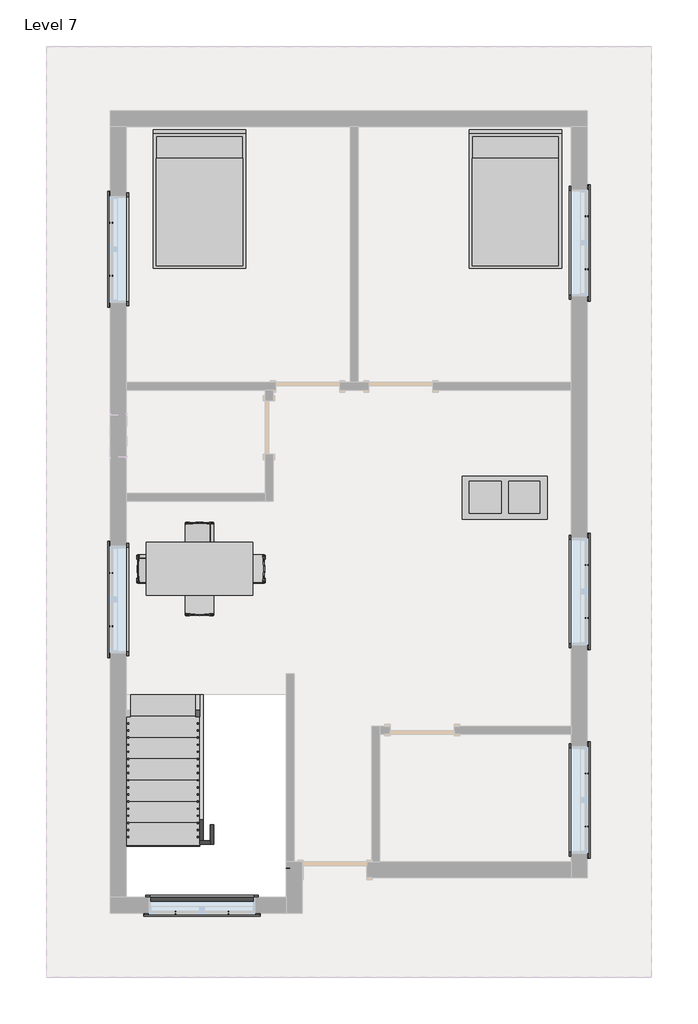
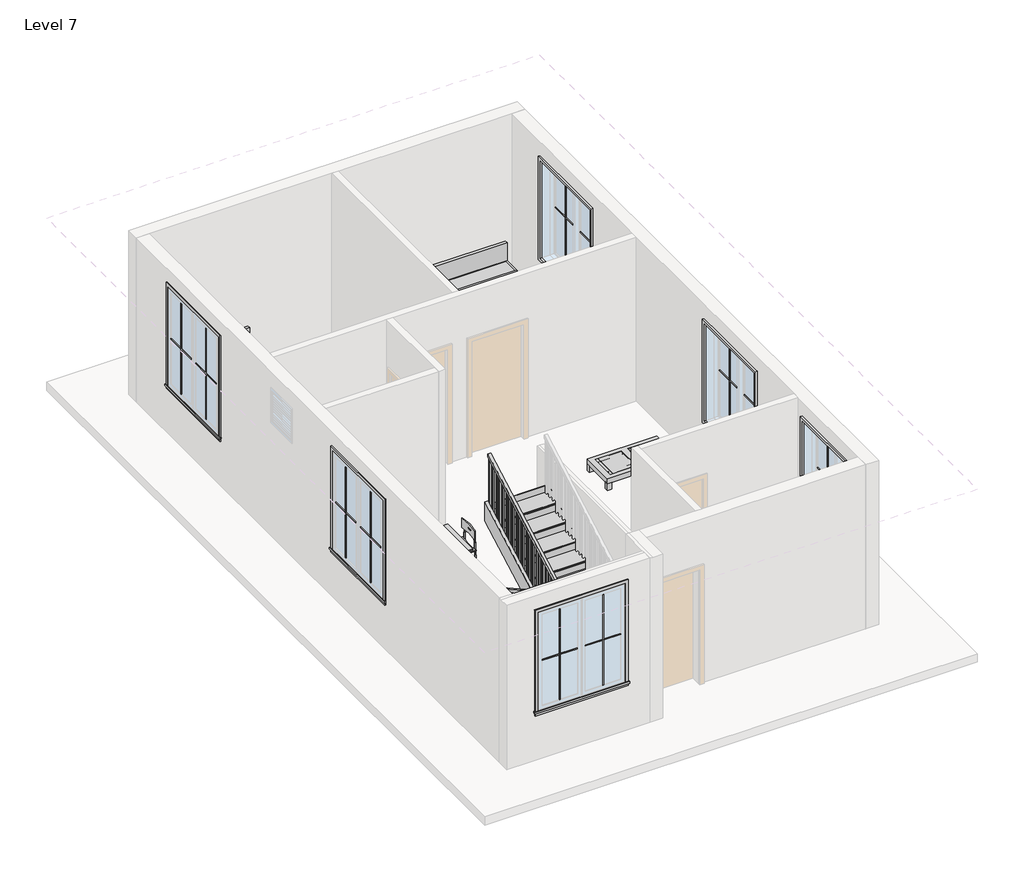
# One storey, part 3 of 3: 25 proxies, 6 members, 3 furniture elements, 1 railing, 1 stair flight.
"""IFC4 building model written with IfcOpenShell, lengths in millimetres."""

from ifc_helpers import new_model, si_unit, frame, origin, place, context, project, spatial, polyline, outline, extrude, faceted_brep, transform, mapped, element, save
from components import muntin_pattern_2x2_muntin_pattern_2x2_f6a80940, muntin_pattern_2x2_muntin_pattern_2x2_09b00a1c, trim_window_exterior_flat_with_sill_698ed857, trim_window_interior_flat_picture_frame_92551a5e, coffee_table_with_brass_mullions_11320_coffee_table_with_5962bef7, bed_17739_bed_17739_15c61121, dining_table_w_chairs_11374_0cdfc61b, stair_flight_c5737279

model = new_model("IFC4")

# Units and contexts
model_context = context("Model", 3, world=origin())
ifc_project = project(units=[si_unit("LENGTHUNIT", "METRE", prefix="MILLI")], contexts=[model_context])

# Site, building, storey
site = spatial("IfcSite", under=ifc_project)
building = spatial("IfcBuilding", under=site)
storey = spatial("IfcBuildingStorey", under=building, Name="Level 7", Elevation=19050.0)

# Proxies
placement = place(None, origin())
muntin_pattern_2x2_muntin_pattern_2x2_shape = muntin_pattern_2x2_muntin_pattern_2x2_f6a80940(model_context)
element("IfcBuildingElementProxy", 1, Name="Muntin Pattern_2x2 : Muntin Pattern_2x2", ObjectType="Muntin Pattern_2x2 : Muntin Pattern_2x2", at=placement, inside=storey, context=model_context, shape_type="MappedRepresentation", body=[
    mapped(muntin_pattern_2x2_muntin_pattern_2x2_shape, transform((-2773.368364, -6686.2830018, 20034.25), x_axis=(-1.0, 0.0, 0.0), y_axis=(0.0, -1.0, 0.0), z_axis=(0.0, 0.0, 1.0))),
])
element("IfcBuildingElementProxy", 2, Name="Muntin Pattern_2x2 : Muntin Pattern_2x2", ObjectType="Muntin Pattern_2x2 : Muntin Pattern_2x2", at=placement, inside=storey, context=model_context, shape_type="MappedRepresentation", body=[
    mapped(muntin_pattern_2x2_muntin_pattern_2x2_shape, transform((2349.494136, -4693.9705018, 20034.25), x_axis=(0.0, -1.0, 0.0), y_axis=(1.0, 0.0, 0.0), z_axis=(0.0, 0.0, 1.0))),
])
element("IfcBuildingElementProxy", 3, Name="Muntin Pattern_2x2 : Muntin Pattern_2x2", ObjectType="Muntin Pattern_2x2 : Muntin Pattern_2x2", at=placement, inside=storey, context=model_context, shape_type="MappedRepresentation", body=[
    mapped(muntin_pattern_2x2_muntin_pattern_2x2_shape, transform((2349.494136, -1712.6455018, 20034.25), x_axis=(0.0, -1.0, 0.0), y_axis=(1.0, 0.0, 0.0), z_axis=(0.0, 0.0, 1.0))),
])
element("IfcBuildingElementProxy", 4, Name="Muntin Pattern_2x2 : Muntin Pattern_2x2", ObjectType="Muntin Pattern_2x2 : Muntin Pattern_2x2", at=placement, inside=storey, context=model_context, shape_type="MappedRepresentation", body=[
    mapped(muntin_pattern_2x2_muntin_pattern_2x2_shape, transform((-4451.355864, -2586.5525081, 20034.25), x_axis=(0.0, 1.0, 0.0), y_axis=(-1.0, 0.0, 0.0), z_axis=(0.0, 0.0, 1.0))),
])
element("IfcBuildingElementProxy", 5, Name="Muntin Pattern_2x2 : Muntin Pattern_2x2", ObjectType="Muntin Pattern_2x2 : Muntin Pattern_2x2", at=placement, inside=storey, context=model_context, shape_type="MappedRepresentation", body=[
    mapped(muntin_pattern_2x2_muntin_pattern_2x2_shape, transform((2349.494136, 3272.1044982, 20034.25), x_axis=(0.0, -1.0, 0.0), y_axis=(1.0, 0.0, 0.0), z_axis=(0.0, 0.0, 1.0))),
])
element("IfcBuildingElementProxy", 6, Name="Muntin Pattern_2x2 : Muntin Pattern_2x2", ObjectType="Muntin Pattern_2x2 : Muntin Pattern_2x2", at=placement, inside=storey, context=model_context, shape_type="MappedRepresentation", body=[
    mapped(muntin_pattern_2x2_muntin_pattern_2x2_shape, transform((-4451.355864, 2421.2162133, 20034.25), x_axis=(0.0, 1.0, 0.0), y_axis=(-1.0, 0.0, 0.0), z_axis=(0.0, 0.0, 1.0))),
])
muntin_pattern_2x2_muntin_pattern_2x2_2_shape = muntin_pattern_2x2_muntin_pattern_2x2_09b00a1c(model_context)
element("IfcBuildingElementProxy", 7, Name="Muntin Pattern_2x2 : Muntin Pattern_2x2", ObjectType="Muntin Pattern_2x2 : Muntin Pattern_2x2", at=placement, inside=storey, context=model_context, shape_type="MappedRepresentation", body=[
    mapped(muntin_pattern_2x2_muntin_pattern_2x2_2_shape, transform((-3532.193364, -6686.2830018, 20034.25), x_axis=(1.0, 0.0, 0.0), y_axis=(0.0, 1.0, 0.0), z_axis=(0.0, 0.0, 1.0))),
])
element("IfcBuildingElementProxy", 8, Name="Muntin Pattern_2x2 : Muntin Pattern_2x2", ObjectType="Muntin Pattern_2x2 : Muntin Pattern_2x2", at=placement, inside=storey, context=model_context, shape_type="MappedRepresentation", body=[
    mapped(muntin_pattern_2x2_muntin_pattern_2x2_2_shape, transform((2349.494136, -5452.7955018, 20034.25), x_axis=(0.0, 1.0, 0.0), y_axis=(-1.0, 0.0, 0.0), z_axis=(0.0, 0.0, 1.0))),
])
element("IfcBuildingElementProxy", 9, Name="Muntin Pattern_2x2 : Muntin Pattern_2x2", ObjectType="Muntin Pattern_2x2 : Muntin Pattern_2x2", at=placement, inside=storey, context=model_context, shape_type="MappedRepresentation", body=[
    mapped(muntin_pattern_2x2_muntin_pattern_2x2_2_shape, transform((2349.494136, -2471.4705018, 20034.25), x_axis=(0.0, 1.0, 0.0), y_axis=(-1.0, 0.0, 0.0), z_axis=(0.0, 0.0, 1.0))),
])
element("IfcBuildingElementProxy", 10, Name="Muntin Pattern_2x2 : Muntin Pattern_2x2", ObjectType="Muntin Pattern_2x2 : Muntin Pattern_2x2", at=placement, inside=storey, context=model_context, shape_type="MappedRepresentation", body=[
    mapped(muntin_pattern_2x2_muntin_pattern_2x2_2_shape, transform((-4451.355864, -1827.7275081, 20034.25), x_axis=(0.0, -1.0, 0.0), y_axis=(1.0, 0.0, 0.0), z_axis=(0.0, 0.0, 1.0))),
])
element("IfcBuildingElementProxy", 11, Name="Muntin Pattern_2x2 : Muntin Pattern_2x2", ObjectType="Muntin Pattern_2x2 : Muntin Pattern_2x2", at=placement, inside=storey, context=model_context, shape_type="MappedRepresentation", body=[
    mapped(muntin_pattern_2x2_muntin_pattern_2x2_2_shape, transform((2349.494136, 2513.2794982, 20034.25), x_axis=(0.0, 1.0, 0.0), y_axis=(-1.0, 0.0, 0.0), z_axis=(0.0, 0.0, 1.0))),
])
element("IfcBuildingElementProxy", 12, Name="Muntin Pattern_2x2 : Muntin Pattern_2x2", ObjectType="Muntin Pattern_2x2 : Muntin Pattern_2x2", at=placement, inside=storey, context=model_context, shape_type="MappedRepresentation", body=[
    mapped(muntin_pattern_2x2_muntin_pattern_2x2_2_shape, transform((-4451.355864, 3180.0412133, 20034.25), x_axis=(0.0, -1.0, 0.0), y_axis=(1.0, 0.0, 0.0), z_axis=(0.0, 0.0, 1.0))),
])
trim_window_exterior_flat_with_sill_shape = trim_window_exterior_flat_with_sill_698ed857(model_context)
element("IfcBuildingElementProxy", 13, Name="Trim-Window-Exterior-Flat : with Sill", ObjectType="Trim-Window-Exterior-Flat : with Sill", at=placement, inside=storey, context=model_context, shape_type="MappedRepresentation", body=[
    mapped(trim_window_exterior_flat_with_sill_shape, transform((-3152.780864, -6695.8080018, 21793.2), x_axis=(1.0, 0.0, 0.0), y_axis=(0.0, 0.0, 1.0), z_axis=(0.0, -1.0, 0.0))),
])
element("IfcBuildingElementProxy", 14, Name="Trim-Window-Exterior-Flat : with Sill", ObjectType="Trim-Window-Exterior-Flat : with Sill", at=placement, inside=storey, context=model_context, shape_type="MappedRepresentation", body=[
    mapped(trim_window_exterior_flat_with_sill_shape, transform((2359.019136, -5073.3830018, 21793.2), x_axis=(0.0, 1.0, 0.0), y_axis=(0.0, 0.0, 1.0), z_axis=(1.0, 0.0, 0.0))),
])
element("IfcBuildingElementProxy", 15, Name="Trim-Window-Exterior-Flat : with Sill", ObjectType="Trim-Window-Exterior-Flat : with Sill", at=placement, inside=storey, context=model_context, shape_type="MappedRepresentation", body=[
    mapped(trim_window_exterior_flat_with_sill_shape, transform((2359.019136, -2092.0580018, 21793.2), x_axis=(0.0, 1.0, 0.0), y_axis=(0.0, 0.0, 1.0), z_axis=(1.0, 0.0, 0.0))),
])
element("IfcBuildingElementProxy", 16, Name="Trim-Window-Exterior-Flat : with Sill", ObjectType="Trim-Window-Exterior-Flat : with Sill", at=placement, inside=storey, context=model_context, shape_type="MappedRepresentation", body=[
    mapped(trim_window_exterior_flat_with_sill_shape, transform((-4460.880864, -2207.1400081, 21793.2), x_axis=(0.0, -1.0, 0.0), y_axis=(0.0, 0.0, 1.0), z_axis=(-1.0, 0.0, 0.0))),
])
element("IfcBuildingElementProxy", 17, Name="Trim-Window-Exterior-Flat : with Sill", ObjectType="Trim-Window-Exterior-Flat : with Sill", at=placement, inside=storey, context=model_context, shape_type="MappedRepresentation", body=[
    mapped(trim_window_exterior_flat_with_sill_shape, transform((2359.019136, 2892.6919982, 21793.2), x_axis=(0.0, 1.0, 0.0), y_axis=(0.0, 0.0, 1.0), z_axis=(1.0, 0.0, 0.0))),
])
element("IfcBuildingElementProxy", 18, Name="Trim-Window-Exterior-Flat : with Sill", ObjectType="Trim-Window-Exterior-Flat : with Sill", at=placement, inside=storey, context=model_context, shape_type="MappedRepresentation", body=[
    mapped(trim_window_exterior_flat_with_sill_shape, transform((-4460.880864, 2800.6287133, 21793.2), x_axis=(0.0, -1.0, 0.0), y_axis=(0.0, 0.0, 1.0), z_axis=(-1.0, 0.0, 0.0))),
])
trim_window_interior_flat_picture_frame_shape = trim_window_interior_flat_picture_frame_92551a5e(model_context)
element("IfcBuildingElementProxy", 19, Name="Trim-Window-Interior-Flat : Picture Frame", ObjectType="Trim-Window-Interior-Flat : Picture Frame", at=placement, inside=storey, context=model_context, shape_type="MappedRepresentation", body=[
    mapped(trim_window_interior_flat_picture_frame_shape, transform((-3152.780864, -6467.2080018, 21793.2), x_axis=(-1.0, 0.0, 0.0), y_axis=(0.0, 0.0, 1.0), z_axis=(0.0, 1.0, 0.0))),
])
element("IfcBuildingElementProxy", 20, Name="Trim-Window-Interior-Flat : Picture Frame", ObjectType="Trim-Window-Interior-Flat : Picture Frame", at=placement, inside=storey, context=model_context, shape_type="MappedRepresentation", body=[
    mapped(trim_window_interior_flat_picture_frame_shape, transform((2130.419136, -5073.3830018, 21793.2), x_axis=(0.0, -1.0, 0.0), y_axis=(0.0, 0.0, 1.0), z_axis=(-1.0, 0.0, 0.0))),
])
element("IfcBuildingElementProxy", 21, Name="Trim-Window-Interior-Flat : Picture Frame", ObjectType="Trim-Window-Interior-Flat : Picture Frame", at=placement, inside=storey, context=model_context, shape_type="MappedRepresentation", body=[
    mapped(trim_window_interior_flat_picture_frame_shape, transform((2130.419136, -2092.0580018, 21793.2), x_axis=(0.0, -1.0, 0.0), y_axis=(0.0, 0.0, 1.0), z_axis=(-1.0, 0.0, 0.0))),
])
element("IfcBuildingElementProxy", 22, Name="Trim-Window-Interior-Flat : Picture Frame", ObjectType="Trim-Window-Interior-Flat : Picture Frame", at=placement, inside=storey, context=model_context, shape_type="MappedRepresentation", body=[
    mapped(trim_window_interior_flat_picture_frame_shape, transform((-4232.280864, -2207.1400081, 21793.2), x_axis=(0.0, 1.0, 0.0), y_axis=(0.0, 0.0, 1.0), z_axis=(1.0, 0.0, 0.0))),
])
element("IfcBuildingElementProxy", 23, Name="Trim-Window-Interior-Flat : Picture Frame", ObjectType="Trim-Window-Interior-Flat : Picture Frame", at=placement, inside=storey, context=model_context, shape_type="MappedRepresentation", body=[
    mapped(trim_window_interior_flat_picture_frame_shape, transform((2130.419136, 2892.6919982, 21793.2), x_axis=(0.0, -1.0, 0.0), y_axis=(0.0, 0.0, 1.0), z_axis=(-1.0, 0.0, 0.0))),
])
element("IfcBuildingElementProxy", 24, Name="Trim-Window-Interior-Flat : Picture Frame", ObjectType="Trim-Window-Interior-Flat : Picture Frame", at=placement, inside=storey, context=model_context, shape_type="MappedRepresentation", body=[
    mapped(trim_window_interior_flat_picture_frame_shape, transform((-4232.280864, 2800.6287133, 21793.2), x_axis=(0.0, 1.0, 0.0), y_axis=(0.0, 0.0, 1.0), z_axis=(1.0, 0.0, 0.0))),
])
coffee_table_with_brass_mullions_11320_coffee_table_with_shape = coffee_table_with_brass_mullions_11320_coffee_table_with_5962bef7(model_context)
element("IfcBuildingElementProxy", 25, Name="coffee_table_with_brass_mullions_11320 : coffee_table_with_brass_mullions_11320", ObjectType="coffee_table_with_brass_mullions_11320 : coffee_table_with_brass_mullions_11320", at=placement, inside=storey, context=model_context, shape_type="MappedRepresentation", body=[
    mapped(coffee_table_with_brass_mullions_11320_coffee_table_with_shape, transform((1812.3816081, -1181.1001099, 19050.0), x_axis=(1.0, 0.0, 0.0), y_axis=(0.0, 1.0, 0.0), z_axis=(0.0, 0.0, 1.0))),
])

# Furniture
bed_17739_bed_17739_shape = bed_17739_bed_17739_15c61121(model_context)
element("IfcFurniture", 26, ObjectType="Bed_17739 : Bed_17739", at=placement, inside=storey, context=model_context, shape_type="MappedRepresentation", body=[
    mapped(bed_17739_bed_17739_shape, transform((1328.5116081, 3496.3098901, 19050.0), x_axis=(1.0, 0.0, 0.0), y_axis=(0.0, 1.0, 0.0), z_axis=(0.0, 0.0, 1.0))),
])
element("IfcFurniture", 27, ObjectType="Bed_17739 : Bed_17739", at=placement, inside=storey, context=model_context, shape_type="MappedRepresentation", body=[
    mapped(bed_17739_bed_17739_shape, transform((-3187.6083919, 3496.3098901, 19050.0), x_axis=(1.0, 0.0, 0.0), y_axis=(0.0, 1.0, 0.0), z_axis=(0.0, 0.0, 1.0))),
])
dining_table_w_chairs_11374_shape = dining_table_w_chairs_11374_0cdfc61b(model_context)
element("IfcFurniture", 28, ObjectType="Dining_Table_w_Chairs_11374", at=placement, inside=storey, context=model_context, shape_type="MappedRepresentation", body=[
    mapped(dining_table_w_chairs_11374_shape, transform((-3205.8741586, -1863.0511877, 19050.0), x_axis=(1.0, 0.0, 0.0), y_axis=(0.0, 1.0, 0.0), z_axis=(0.0, 0.0, 1.0))),
])

# Members
element("IfcMember", 29, ObjectType="Stringer - 2\" Width", at=placement, inside=storey, context=model_context, shape_type="SweptSolid", body=[
    extrude(outline(polyline([(-3571.6080018, 19257.5983948), (-3571.6080018, 19050.0), (-3825.5525046, 19050.0), (-5654.4080018, 20066.0308318), (-5654.4080018, 20414.7095059), (-3571.6080018, 19257.5983948)])), frame((-3187.6083919, 0.0, 0.0), z_axis=(1.0, 0.0, 0.0), x_axis=(0.0, 1.0, 0.0)), (0.0, 0.0, 1.0), 50.8),
])
element("IfcMember", 30, ObjectType="Stringer - 2\" Width", at=placement, inside=storey, context=model_context, shape_type="SweptSolid", body=[
    extrude(outline(polyline([(-3187.6083919, -5705.2080018), (-3187.6083919, -5654.4080018), (-3035.2083919, -5654.4080018), (-3035.2083919, -5705.2080018), (-3187.6083919, -5705.2080018)])), frame((0.0, 0.0, 20176.0666667), z_axis=(0.0, 0.0, 1.0), x_axis=(1.0, 0.0, 0.0)), (0.0, 0.0, 1.0), 304.8),
])
element("IfcMember", 31, ObjectType="Stringer - 2\" Width", at=placement, inside=storey, context=model_context, shape_type="SweptSolid", body=[
    extrude(outline(polyline([(-5705.2080018, 20176.0666667), (-5705.2080018, 20442.9317281), (-3571.6080018, 21628.2650614), (-3571.6080018, 21279.5863873), (-5557.943499, 20176.0666667), (-5705.2080018, 20176.0666667)])), frame((-3035.2083919, 0.0, 0.0), z_axis=(1.0, 0.0, 0.0), x_axis=(0.0, 1.0, 0.0)), (0.0, 0.0, 1.0), 50.8),
])
element("IfcMember", 32, ObjectType="Stringer - 2\" Width", at=placement, inside=storey, context=model_context, shape_type="SweptSolid", body=[
    extrude(outline(polyline([(-3571.6080018, 19257.5983948), (-3571.6080018, 19050.0), (-3825.5525046, 19050.0), (-6401.1125046, 20480.8666667), (-5773.4908912, 20480.8666667), (-3571.6080018, 19257.5983948)])), frame((-4283.080864, 0.0, 0.0), z_axis=(1.0, 0.0, 0.0), x_axis=(0.0, 1.0, 0.0)), (0.0, 0.0, 1.0), 50.8),
])
element("IfcMember", 33, ObjectType="Stringer - 2\" Width", at=placement, inside=storey, context=model_context, shape_type="SweptSolid", body=[
    extrude(outline(polyline([(-4283.080864, -6518.0080018), (-4283.080864, -6467.2080018), (-1946.280864, -6467.2080018), (-1946.280864, -6518.0080018), (-4283.080864, -6518.0080018)])), frame((0.0, 0.0, 20176.0666667), z_axis=(0.0, 0.0, 1.0), x_axis=(1.0, 0.0, 0.0)), (0.0, 0.0, 1.0), 304.8),
])
element("IfcMember", 34, ObjectType="Stringer - 2\" Width", at=placement, inside=storey, context=model_context, shape_type="SweptSolid", body=[
    extrude(outline(polyline([(-6185.5651124, 20176.0666667), (-3571.6080018, 21628.2650614), (-3571.6080018, 21279.5863873), (-5557.943499, 20176.0666667), (-6185.5651124, 20176.0666667)])), frame((-1946.280864, 0.0, 0.0), z_axis=(1.0, 0.0, 0.0), x_axis=(0.0, 1.0, 0.0)), (0.0, 0.0, 1.0), 50.8),
])

# Railing
element("IfcRailing", 35, ObjectType="Handrail - Rectangular", at=placement, inside=storey, context=model_context, shape_type="SolidModel", body=[
    faceted_brep([(-3187.6083919, -3571.6080018, 20133.7333333), (-3187.6083919, -3571.6080018, 20075.620221), (-3238.4083919, -3571.6080018, 20075.620221), (-3238.4083919, -3571.6080018, 20133.7333333), (-3187.6083919, -5629.0080018, 21276.7333333), (-3187.6083919, -5679.8080018, 21246.8424432), (-3238.4083919, -5679.8080018, 21246.8424432), (-3238.4083919, -5629.0080018, 21276.7333333), (-3187.6083919, -5629.0080018, 21319.0666667), (-3187.6083919, -5679.8080018, 21268.2666667), (-3238.4083919, -5679.8080018, 21268.2666667), (-3238.4083919, -5629.0080018, 21319.0666667), (-3187.6083919, -5705.2080018, 21319.0666667), (-3187.6083919, -5705.2080018, 21268.2666667), (-3238.4083919, -5756.0080018, 21268.2666667), (-3238.4083919, -5756.0080018, 21319.0666667), (-3111.4083919, -5705.2080018, 21319.0666667), (-3111.4083919, -5705.2080018, 21268.2666667), (-3111.4083919, -5756.0080018, 21268.2666667), (-3111.4083919, -5756.0080018, 21319.0666667), (-3060.6083919, -5705.2080018, 21319.0666667), (-3009.8083919, -5705.2080018, 21268.2666667), (-3009.8083919, -5756.0080018, 21268.2666667), (-3060.6083919, -5756.0080018, 21319.0666667), (-3060.6083919, -5705.2080018, 21361.4), (-3009.8083919, -5705.2080018, 21310.6), (-3009.8083919, -5756.0080018, 21310.6), (-3060.6083919, -5756.0080018, 21361.4), (-2984.4083919, -5705.2080018, 21361.4), (-2984.4083919, -5705.2080018, 21310.6), (-2933.6083919, -5756.0080018, 21310.6), (-2933.6083919, -5756.0080018, 21361.4), (-2984.4083919, -5629.0080018, 21361.4), (-2984.4083919, -5615.8443995, 21310.6), (-2933.6083919, -5615.8443995, 21310.6), (-2933.6083919, -5629.0080018, 21361.4), (-2984.4083919, -3571.6080018, 22504.4), (-2933.6083919, -3571.6080018, 22504.4), (-2933.6083919, -3571.6080018, 22446.2868876), (-2984.4083919, -3571.6080018, 22446.2868876)], [[[0, 1, 2, 3]], [[1, 0, 4, 5]], [[2, 1, 5, 6]], [[3, 2, 6, 7]], [[0, 3, 7, 4]], [[5, 4, 8, 9]], [[6, 5, 9, 10]], [[7, 6, 10, 11]], [[4, 7, 11, 8]], [[9, 8, 12, 13]], [[10, 9, 13, 14]], [[11, 10, 14, 15]], [[8, 11, 15, 12]], [[13, 12, 16, 17]], [[14, 13, 17, 18]], [[15, 14, 18, 19]], [[12, 15, 19, 16]], [[17, 16, 20, 21]], [[18, 17, 21, 22]], [[19, 18, 22, 23]], [[16, 19, 23, 20]], [[21, 20, 24, 25]], [[22, 21, 25, 26]], [[23, 22, 26, 27]], [[20, 23, 27, 24]], [[25, 24, 28, 29]], [[26, 25, 29, 30]], [[27, 26, 30, 31]], [[24, 27, 31, 28]], [[29, 28, 32, 33]], [[30, 29, 33, 34]], [[31, 30, 34, 35]], [[28, 31, 35, 32]], [[36, 37, 38, 39]], [[33, 32, 36, 39]], [[34, 33, 39, 38]], [[35, 34, 38, 37]], [[32, 35, 37, 36]]]),
    extrude(outline(polyline([(-3587.4830018, 22437.4674432), (-3587.4830018, 21420.6666667), (-3606.5330018, 21420.6666667), (-3606.5330018, 22426.8841099), (-3587.4830018, 22437.4674432)])), frame((-2968.5333919, 0.0, 0.0), z_axis=(1.0, 0.0, 0.0), x_axis=(0.0, 1.0, 0.0)), (0.0, 0.0, 1.0), 19.05),
    extrude(outline(polyline([(-3689.0830018, 22381.0229988), (-3689.0830018, 21420.6666667), (-3708.1330018, 21420.6666667), (-3708.1330018, 22370.4396654), (-3689.0830018, 22381.0229988)])), frame((-2968.5333919, 0.0, 0.0), z_axis=(1.0, 0.0, 0.0), x_axis=(0.0, 1.0, 0.0)), (0.0, 0.0, 1.0), 19.05),
    extrude(outline(polyline([(-3790.6830018, 22324.5785543), (-3790.6830018, 21420.6666667), (-3809.7330018, 21420.6666667), (-3809.7330018, 22313.995221), (-3790.6830018, 22324.5785543)])), frame((-2968.5333919, 0.0, 0.0), z_axis=(1.0, 0.0, 0.0), x_axis=(0.0, 1.0, 0.0)), (0.0, 0.0, 1.0), 19.05),
    extrude(outline(polyline([(-3892.2830018, 22268.1341099), (-3892.2830018, 21251.3333333), (-3911.3330018, 21251.3333333), (-3911.3330018, 22257.5507765), (-3892.2830018, 22268.1341099)])), frame((-2968.5333919, 0.0, 0.0), z_axis=(1.0, 0.0, 0.0), x_axis=(0.0, 1.0, 0.0)), (0.0, 0.0, 1.0), 19.05),
    extrude(outline(polyline([(-3993.8830018, 22211.6896654), (-3993.8830018, 21251.3333333), (-4012.9330018, 21251.3333333), (-4012.9330018, 22201.1063321), (-3993.8830018, 22211.6896654)])), frame((-2968.5333919, 0.0, 0.0), z_axis=(1.0, 0.0, 0.0), x_axis=(0.0, 1.0, 0.0)), (0.0, 0.0, 1.0), 19.05),
    extrude(outline(polyline([(-4095.4830018, 22155.245221), (-4095.4830018, 21251.3333333), (-4114.5330018, 21251.3333333), (-4114.5330018, 22144.6618876), (-4095.4830018, 22155.245221)])), frame((-2968.5333919, 0.0, 0.0), z_axis=(1.0, 0.0, 0.0), x_axis=(0.0, 1.0, 0.0)), (0.0, 0.0, 1.0), 19.05),
    extrude(outline(polyline([(-4197.0830018, 22098.8007765), (-4197.0830018, 21082.0), (-4216.1330018, 21082.0), (-4216.1330018, 22088.2174432), (-4197.0830018, 22098.8007765)])), frame((-2968.5333919, 0.0, 0.0), z_axis=(1.0, 0.0, 0.0), x_axis=(0.0, 1.0, 0.0)), (0.0, 0.0, 1.0), 19.05),
    extrude(outline(polyline([(-4298.6830018, 22042.3563321), (-4298.6830018, 21082.0), (-4317.7330018, 21082.0), (-4317.7330018, 22031.7729988), (-4298.6830018, 22042.3563321)])), frame((-2968.5333919, 0.0, 0.0), z_axis=(1.0, 0.0, 0.0), x_axis=(0.0, 1.0, 0.0)), (0.0, 0.0, 1.0), 19.05),
    extrude(outline(polyline([(-4400.2830018, 21985.9118876), (-4400.2830018, 21082.0), (-4419.3330018, 21082.0), (-4419.3330018, 21975.3285543), (-4400.2830018, 21985.9118876)])), frame((-2968.5333919, 0.0, 0.0), z_axis=(1.0, 0.0, 0.0), x_axis=(0.0, 1.0, 0.0)), (0.0, 0.0, 1.0), 19.05),
    extrude(outline(polyline([(-4501.8830018, 21929.4674432), (-4501.8830018, 20912.6666667), (-4520.9330018, 20912.6666667), (-4520.9330018, 21918.8841099), (-4501.8830018, 21929.4674432)])), frame((-2968.5333919, 0.0, 0.0), z_axis=(1.0, 0.0, 0.0), x_axis=(0.0, 1.0, 0.0)), (0.0, 0.0, 1.0), 19.05),
    extrude(outline(polyline([(-4603.4830018, 21873.0229988), (-4603.4830018, 20912.6666667), (-4622.5330018, 20912.6666667), (-4622.5330018, 21862.4396654), (-4603.4830018, 21873.0229988)])), frame((-2968.5333919, 0.0, 0.0), z_axis=(1.0, 0.0, 0.0), x_axis=(0.0, 1.0, 0.0)), (0.0, 0.0, 1.0), 19.05),
    extrude(outline(polyline([(-4705.0830018, 21816.5785543), (-4705.0830018, 20912.6666667), (-4724.1330018, 20912.6666667), (-4724.1330018, 21805.995221), (-4705.0830018, 21816.5785543)])), frame((-2968.5333919, 0.0, 0.0), z_axis=(1.0, 0.0, 0.0), x_axis=(0.0, 1.0, 0.0)), (0.0, 0.0, 1.0), 19.05),
    extrude(outline(polyline([(-4806.6830018, 21760.1341099), (-4806.6830018, 20743.3333333), (-4825.7330018, 20743.3333333), (-4825.7330018, 21749.5507765), (-4806.6830018, 21760.1341099)])), frame((-2968.5333919, 0.0, 0.0), z_axis=(1.0, 0.0, 0.0), x_axis=(0.0, 1.0, 0.0)), (0.0, 0.0, 1.0), 19.05),
    extrude(outline(polyline([(-4908.2830018, 21703.6896654), (-4908.2830018, 20743.3333333), (-4927.3330018, 20743.3333333), (-4927.3330018, 21693.1063321), (-4908.2830018, 21703.6896654)])), frame((-2968.5333919, 0.0, 0.0), z_axis=(1.0, 0.0, 0.0), x_axis=(0.0, 1.0, 0.0)), (0.0, 0.0, 1.0), 19.05),
    extrude(outline(polyline([(-5009.8830018, 21647.245221), (-5009.8830018, 20743.3333333), (-5028.9330018, 20743.3333333), (-5028.9330018, 21636.6618876), (-5009.8830018, 21647.245221)])), frame((-2968.5333919, 0.0, 0.0), z_axis=(1.0, 0.0, 0.0), x_axis=(0.0, 1.0, 0.0)), (0.0, 0.0, 1.0), 19.05),
    extrude(outline(polyline([(-5111.4830018, 21590.8007765), (-5111.4830018, 20574.0), (-5130.5330018, 20574.0), (-5130.5330018, 21580.2174432), (-5111.4830018, 21590.8007765)])), frame((-2968.5333919, 0.0, 0.0), z_axis=(1.0, 0.0, 0.0), x_axis=(0.0, 1.0, 0.0)), (0.0, 0.0, 1.0), 19.05),
    extrude(outline(polyline([(-5213.0830018, 21534.3563321), (-5213.0830018, 20574.0), (-5232.1330018, 20574.0), (-5232.1330018, 21523.7729988), (-5213.0830018, 21534.3563321)])), frame((-2968.5333919, 0.0, 0.0), z_axis=(1.0, 0.0, 0.0), x_axis=(0.0, 1.0, 0.0)), (0.0, 0.0, 1.0), 19.05),
    extrude(outline(polyline([(-5314.6830018, 21477.9118876), (-5314.6830018, 20574.0), (-5333.7330018, 20574.0), (-5333.7330018, 21467.3285543), (-5314.6830018, 21477.9118876)])), frame((-2968.5333919, 0.0, 0.0), z_axis=(1.0, 0.0, 0.0), x_axis=(0.0, 1.0, 0.0)), (0.0, 0.0, 1.0), 19.05),
    extrude(outline(polyline([(-5416.2830018, 21421.4674432), (-5416.2830018, 20404.6666667), (-5435.3330018, 20404.6666667), (-5435.3330018, 21410.8841099), (-5416.2830018, 21421.4674432)])), frame((-2968.5333919, 0.0, 0.0), z_axis=(1.0, 0.0, 0.0), x_axis=(0.0, 1.0, 0.0)), (0.0, 0.0, 1.0), 19.05),
    extrude(outline(polyline([(-5517.8830018, 21365.0229988), (-5517.8830018, 20404.6666667), (-5536.9330018, 20404.6666667), (-5536.9330018, 21354.4396654), (-5517.8830018, 21365.0229988)])), frame((-2968.5333919, 0.0, 0.0), z_axis=(1.0, 0.0, 0.0), x_axis=(0.0, 1.0, 0.0)), (0.0, 0.0, 1.0), 19.05),
    extrude(outline(polyline([(-5619.4830018, 21308.5785543), (-5619.4830018, 20404.6666667), (-5638.5330018, 20404.6666667), (-5638.5330018, 21297.995221), (-5619.4830018, 21308.5785543)])), frame((-2968.5333919, 0.0, 0.0), z_axis=(1.0, 0.0, 0.0), x_axis=(0.0, 1.0, 0.0)), (0.0, 0.0, 1.0), 19.05),
    extrude(outline(polyline([(-3019.3333919, -5721.0830018), (-3000.2833919, -5721.0830018), (-3000.2833919, -5740.1330018), (-3019.3333919, -5740.1330018), (-3019.3333919, -5721.0830018)])), frame((0.0, 0.0, 20404.6666667), z_axis=(0.0, 0.0, 1.0), x_axis=(1.0, 0.0, 0.0)), (0.0, 0.0, 1.0), 905.9333333),
    extrude(outline(polyline([(-3120.9333919, -5721.0830018), (-3101.8833919, -5721.0830018), (-3101.8833919, -5740.1330018), (-3120.9333919, -5740.1330018), (-3120.9333919, -5721.0830018)])), frame((0.0, 0.0, 20404.6666667), z_axis=(0.0, 0.0, 1.0), x_axis=(1.0, 0.0, 0.0)), (0.0, 0.0, 1.0), 863.6),
    extrude(outline(polyline([(-3203.4833919, -5695.6830018), (-3203.4833919, -5714.7330018), (-3222.5333919, -5714.7330018), (-3222.5333919, -5695.6830018), (-3203.4833919, -5695.6830018)])), frame((0.0, 0.0, 20404.6666667), z_axis=(0.0, 0.0, 1.0), x_axis=(1.0, 0.0, 0.0)), (0.0, 0.0, 1.0), 863.6),
    extrude(outline(polyline([(-5594.0830018, 21199.2174432), (-5594.0830018, 20235.3333333), (-5613.1330018, 20235.3333333), (-5613.1330018, 21209.8007765), (-5594.0830018, 21199.2174432)])), frame((-3222.5333919, 0.0, 0.0), z_axis=(1.0, 0.0, 0.0), x_axis=(0.0, 1.0, 0.0)), (0.0, 0.0, 1.0), 19.05),
    extrude(outline(polyline([(-5492.4830018, 21142.7729988), (-5492.4830018, 20235.3333333), (-5511.5330018, 20235.3333333), (-5511.5330018, 21153.3563321), (-5492.4830018, 21142.7729988)])), frame((-3222.5333919, 0.0, 0.0), z_axis=(1.0, 0.0, 0.0), x_axis=(0.0, 1.0, 0.0)), (0.0, 0.0, 1.0), 19.05),
    extrude(outline(polyline([(-5390.8830018, 21086.3285543), (-5390.8830018, 20235.3333333), (-5409.9330018, 20235.3333333), (-5409.9330018, 21096.9118876), (-5390.8830018, 21086.3285543)])), frame((-3222.5333919, 0.0, 0.0), z_axis=(1.0, 0.0, 0.0), x_axis=(0.0, 1.0, 0.0)), (0.0, 0.0, 1.0), 19.05),
    extrude(outline(polyline([(-5289.2830018, 21029.8841099), (-5289.2830018, 20066.0), (-5308.3330018, 20066.0), (-5308.3330018, 21040.4674432), (-5289.2830018, 21029.8841099)])), frame((-3222.5333919, 0.0, 0.0), z_axis=(1.0, 0.0, 0.0), x_axis=(0.0, 1.0, 0.0)), (0.0, 0.0, 1.0), 19.05),
    extrude(outline(polyline([(-5187.6830018, 20973.4396654), (-5187.6830018, 20066.0), (-5206.7330018, 20066.0), (-5206.7330018, 20984.0229988), (-5187.6830018, 20973.4396654)])), frame((-3222.5333919, 0.0, 0.0), z_axis=(1.0, 0.0, 0.0), x_axis=(0.0, 1.0, 0.0)), (0.0, 0.0, 1.0), 19.05),
    extrude(outline(polyline([(-5086.0830018, 20916.995221), (-5086.0830018, 20066.0), (-5105.1330018, 20066.0), (-5105.1330018, 20927.5785543), (-5086.0830018, 20916.995221)])), frame((-3222.5333919, 0.0, 0.0), z_axis=(1.0, 0.0, 0.0), x_axis=(0.0, 1.0, 0.0)), (0.0, 0.0, 1.0), 19.05),
    extrude(outline(polyline([(-4984.4830018, 20860.5507765), (-4984.4830018, 19896.6666667), (-5003.5330018, 19896.6666667), (-5003.5330018, 20871.1341099), (-4984.4830018, 20860.5507765)])), frame((-3222.5333919, 0.0, 0.0), z_axis=(1.0, 0.0, 0.0), x_axis=(0.0, 1.0, 0.0)), (0.0, 0.0, 1.0), 19.05),
    extrude(outline(polyline([(-4882.8830018, 20804.1063321), (-4882.8830018, 19896.6666667), (-4901.9330018, 19896.6666667), (-4901.9330018, 20814.6896654), (-4882.8830018, 20804.1063321)])), frame((-3222.5333919, 0.0, 0.0), z_axis=(1.0, 0.0, 0.0), x_axis=(0.0, 1.0, 0.0)), (0.0, 0.0, 1.0), 19.05),
    extrude(outline(polyline([(-4781.2830018, 20747.6618876), (-4781.2830018, 19896.6666667), (-4800.3330018, 19896.6666667), (-4800.3330018, 20758.245221), (-4781.2830018, 20747.6618876)])), frame((-3222.5333919, 0.0, 0.0), z_axis=(1.0, 0.0, 0.0), x_axis=(0.0, 1.0, 0.0)), (0.0, 0.0, 1.0), 19.05),
    extrude(outline(polyline([(-4679.6830018, 20691.2174432), (-4679.6830018, 19727.3333333), (-4698.7330018, 19727.3333333), (-4698.7330018, 20701.8007765), (-4679.6830018, 20691.2174432)])), frame((-3222.5333919, 0.0, 0.0), z_axis=(1.0, 0.0, 0.0), x_axis=(0.0, 1.0, 0.0)), (0.0, 0.0, 1.0), 19.05),
    extrude(outline(polyline([(-4578.0830018, 20634.7729988), (-4578.0830018, 19727.3333333), (-4597.1330018, 19727.3333333), (-4597.1330018, 20645.3563321), (-4578.0830018, 20634.7729988)])), frame((-3222.5333919, 0.0, 0.0), z_axis=(1.0, 0.0, 0.0), x_axis=(0.0, 1.0, 0.0)), (0.0, 0.0, 1.0), 19.05),
    extrude(outline(polyline([(-4476.4830018, 20578.3285543), (-4476.4830018, 19727.3333333), (-4495.5330018, 19727.3333333), (-4495.5330018, 20588.9118876), (-4476.4830018, 20578.3285543)])), frame((-3222.5333919, 0.0, 0.0), z_axis=(1.0, 0.0, 0.0), x_axis=(0.0, 1.0, 0.0)), (0.0, 0.0, 1.0), 19.05),
    extrude(outline(polyline([(-4374.8830018, 20521.8841099), (-4374.8830018, 19558.0), (-4393.9330018, 19558.0), (-4393.9330018, 20532.4674432), (-4374.8830018, 20521.8841099)])), frame((-3222.5333919, 0.0, 0.0), z_axis=(1.0, 0.0, 0.0), x_axis=(0.0, 1.0, 0.0)), (0.0, 0.0, 1.0), 19.05),
    extrude(outline(polyline([(-4273.2830018, 20465.4396654), (-4273.2830018, 19558.0), (-4292.3330018, 19558.0), (-4292.3330018, 20476.0229988), (-4273.2830018, 20465.4396654)])), frame((-3222.5333919, 0.0, 0.0), z_axis=(1.0, 0.0, 0.0), x_axis=(0.0, 1.0, 0.0)), (0.0, 0.0, 1.0), 19.05),
    extrude(outline(polyline([(-4171.6830018, 20408.995221), (-4171.6830018, 19558.0), (-4190.7330018, 19558.0), (-4190.7330018, 20419.5785543), (-4171.6830018, 20408.995221)])), frame((-3222.5333919, 0.0, 0.0), z_axis=(1.0, 0.0, 0.0), x_axis=(0.0, 1.0, 0.0)), (0.0, 0.0, 1.0), 19.05),
    extrude(outline(polyline([(-4070.0830018, 20352.5507765), (-4070.0830018, 19388.6666667), (-4089.1330018, 19388.6666667), (-4089.1330018, 20363.1341099), (-4070.0830018, 20352.5507765)])), frame((-3222.5333919, 0.0, 0.0), z_axis=(1.0, 0.0, 0.0), x_axis=(0.0, 1.0, 0.0)), (0.0, 0.0, 1.0), 19.05),
    extrude(outline(polyline([(-3968.4830018, 20296.1063321), (-3968.4830018, 19388.6666667), (-3987.5330018, 19388.6666667), (-3987.5330018, 20306.6896654), (-3968.4830018, 20296.1063321)])), frame((-3222.5333919, 0.0, 0.0), z_axis=(1.0, 0.0, 0.0), x_axis=(0.0, 1.0, 0.0)), (0.0, 0.0, 1.0), 19.05),
    extrude(outline(polyline([(-3866.8830018, 20239.6618876), (-3866.8830018, 19388.6666667), (-3885.9330018, 19388.6666667), (-3885.9330018, 20250.245221), (-3866.8830018, 20239.6618876)])), frame((-3222.5333919, 0.0, 0.0), z_axis=(1.0, 0.0, 0.0), x_axis=(0.0, 1.0, 0.0)), (0.0, 0.0, 1.0), 19.05),
    extrude(outline(polyline([(-3765.2830018, 20183.2174432), (-3765.2830018, 19219.3333333), (-3784.3330018, 19219.3333333), (-3784.3330018, 20193.8007765), (-3765.2830018, 20183.2174432)])), frame((-3222.5333919, 0.0, 0.0), z_axis=(1.0, 0.0, 0.0), x_axis=(0.0, 1.0, 0.0)), (0.0, 0.0, 1.0), 19.05),
    extrude(outline(polyline([(-3663.6830018, 20126.7729988), (-3663.6830018, 19219.3333333), (-3682.7330018, 19219.3333333), (-3682.7330018, 20137.3563321), (-3663.6830018, 20126.7729988)])), frame((-3222.5333919, 0.0, 0.0), z_axis=(1.0, 0.0, 0.0), x_axis=(0.0, 1.0, 0.0)), (0.0, 0.0, 1.0), 19.05),
    extrude(outline(polyline([(-2968.5333919, -5721.0830018), (-2949.4833919, -5721.0830018), (-2949.4833919, -5740.1330018), (-2968.5333919, -5740.1330018), (-2968.5333919, -5721.0830018)])), frame((0.0, 0.0, 20404.6666667), z_axis=(0.0, 0.0, 1.0), x_axis=(1.0, 0.0, 0.0)), (0.0, 0.0, 1.0), 905.9333333),
    extrude(outline(polyline([(-3203.4833919, -5721.0830018), (-3203.4833919, -5740.1330018), (-3222.5333919, -5740.1330018), (-3222.5333919, -5721.0830018), (-3203.4833919, -5721.0830018)])), frame((0.0, 0.0, 20404.6666667), z_axis=(0.0, 0.0, 1.0), x_axis=(1.0, 0.0, 0.0)), (0.0, 0.0, 1.0), 863.6),
    extrude(outline(polyline([(-3571.6080018, 22446.2868876), (-3571.6080018, 21420.6666667), (-3590.6580018, 21420.6666667), (-3590.6580018, 22435.7035543), (-3571.6080018, 22446.2868876)])), frame((-2968.5333919, 0.0, 0.0), z_axis=(1.0, 0.0, 0.0), x_axis=(0.0, 1.0, 0.0)), (0.0, 0.0, 1.0), 19.05),
    extrude(outline(polyline([(-3571.6080018, 20075.620221), (-3571.6080018, 19219.3333333), (-3590.6580018, 19219.3333333), (-3590.6580018, 20086.2035543), (-3571.6080018, 20075.620221)])), frame((-3222.5333919, 0.0, 0.0), z_axis=(1.0, 0.0, 0.0), x_axis=(0.0, 1.0, 0.0)), (0.0, 0.0, 1.0), 19.05),
])

# Stair flight
stair_flight_shape = stair_flight_c5737279(model_context)
element("IfcStairFlight", 36, ObjectType="2\" Tread 1\" Nosing 1/4\" Riser", at=placement, inside=storey, context=model_context, shape_type="MappedRepresentation", body=[
    mapped(stair_flight_shape, transform((0.0, 0.0, 0.0), x_axis=(1.0, 0.0, 0.0), y_axis=(0.0, 1.0, 0.0), z_axis=(0.0, 0.0, 1.0))),
])

save(model, "model.ifc")

# Revit data of these elements
# Type "Muntin Pattern_2x2 : Muntin Pattern_2x2"
#   Width [instance default] = 4' - 0"
#   Thickness = 0' - 0 1/2"
#   Height [instance default] = 4' - 0"
#   Distance = 0' - 0 3/4"
#   Interior Material [instance default] = none
#   Exterior Material [instance default] = none
#   Default Elevation = 0
# Type "Trim-Window-Exterior-Flat : with Sill"
#   Trim Width = 0' - 2 1/4"
#   Trim Thickness_Picture Frame = 0' - 1 1/4"
#   Trim Thickness_with Sill = 0' - 0 3/4"
#   Sill Thickness = 0' - 1 1/4"
#   Opening Width [instance default] = 2' - 0"
#   Opening Height [instance default] = 3' - 0"
#   Default Elevation = 4' - 0"
#   Sill = yes
#   Picture Frame = no
#   Trim Material [instance default] = none
# Type "Trim-Window-Interior-Flat : Picture Frame"
#   Trim Thickness_Picture Frame = 0' - 1 1/4"
#   Trim Width = 0' - 2 1/4"
#   Trim Thickness_with Sill = 0' - 0 3/4"
#   Sill Thickness = 0' - 1 1/4"
#   Opening Width [instance default] = 2' - 0"
#   Opening Height [instance default] = 3' - 0"
#   Default Elevation = 4' - 0"
#   Sill = no
#   Picture Frame = yes
#   Trim Material [instance default] = none
# Type "coffee_table_with_brass_mullions_11320 : coffee_table_with_brass_mullions_11320"
#   Default Elevation = 0
# Type "Bed_17739 : Bed_17739"
#   Default Elevation = 0
# Type "Dining_Table_w_Chairs_11374"
#   Default Elevation = 0
#   Assembly Code = ""
# Type "Handrail - Rectangular"
#   Assembly Code = "C2010400"
#   built-in parameter 1008612 = 0.0416667 (stored number, unit not read)
#   built-in parameter 1008611 = 0.0416667 (stored number, unit not read)
#   built-in parameter 1008609 = 0.333333 (stored number, unit not read)
#   built-in parameter 1008604 = 0.166667 (stored number, unit not read)
#   built-in parameter 1008603 = 0.166667 (stored number, unit not read)
#   Railing Height = 3' - 0"
#   built-in parameter 1008630 = 2
#   built-in parameter 1008610 = 2
#   built-in parameter 1008618 = Baluster - Square : 3/4"
# Elements 1, 2, 3, 4, 5, 6, 7, 8, 9, 10, 11, 12 (IfcBuildingElementProxy, "Muntin Pattern_2x2 : Muntin Pattern_2x2")
#   Width = 2' - 0 5/8"
#   Height = 5' - 6 1/2"
#   Interior Material = Wood - Stained
#   Exterior Material = Clad - White
#   Phase Created = New Construction
#   Materials on its faces: "Clad - White", "Wood - Stained"
# Elements 13, 14, 15, 16, 17, 18 (IfcBuildingElementProxy, "Trim-Window-Exterior-Flat : with Sill")
#   Opening Width = 5' - 0"
#   Opening Height = 6' - 0"
#   Trim Material = Clad - White
#   Phase Created = New Construction
#   Materials on its faces: "Clad - White"
# Elements 19, 20, 21, 22, 23, 24 (IfcBuildingElementProxy, "Trim-Window-Interior-Flat : Picture Frame")
#   Opening Width = 5' - 0"
#   Opening Height = 6' - 0"
#   Trim Material = Wood - Stained
#   Phase Created = New Construction
#   Materials on its faces: "Wood - Stained"
# Element 25 (IfcBuildingElementProxy, "coffee_table_with_brass_mullions_11320 : coffee_table_with_brass_mullions_11320")
#   Phase Created = New Construction
#   Materials on its faces: "Default Wall", "TABLE", "Glass", "Default"
# Elements 26, 27 (IfcFurniture, "Bed_17739 : Bed_17739")
#   Phase Created = New Construction
#   Materials on its faces: "legs", "sheets", "bed frame", "Blanket"
# Element 28 (IfcFurniture, "Dining_Table_w_Chairs_11374")
#   Phase Created = New Construction
# Elements 29, 30, 31, 32, 33, 34 (IfcMember, "Stringer - 2\" Width")
#   Phase Created = New Construction
# Element 35 (IfcRailing, "Handrail - Rectangular")
#   Phase Created = New Construction
# Element 36 (IfcStairFlight, "2\" Tread 1\" Nosing 1/4\" Riser")
#   Phase Created = New Construction
# Materials
#   "Clad - White": class "Wood", colour RGB 242 242 238, transparency 0, Cost = 0
#   "Wood - Stained": class "Wood", colour RGB 224 178 126, transparency 0, Cost = 0
#   "Default Wall": colour RGB 128 128 128, transparency 0, Cost = 0
#   "TABLE": class "Generic", colour RGB 120 120 120, transparency 0, Cost = 0
#   "Glass": class "Glass", colour RGB 0 128 192, transparency 0.75, Description = "Soda Lime Glass", Cost = 0
#   "Default": colour RGB 127 127 127, transparency 0, Cost = 0
#   "legs": colour RGB 90 73 37, transparency 0, Cost = 0
#   "sheets": colour RGB 200 195 176, transparency 0, Cost = 0
#   "bed frame": colour RGB 90 73 37, transparency 0, Cost = 0
#   "Blanket": class "System", colour RGB 59 0 1, transparency 0, Cost = 0
